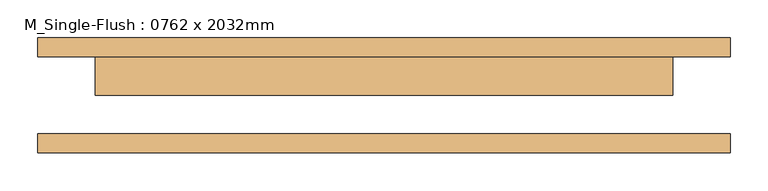
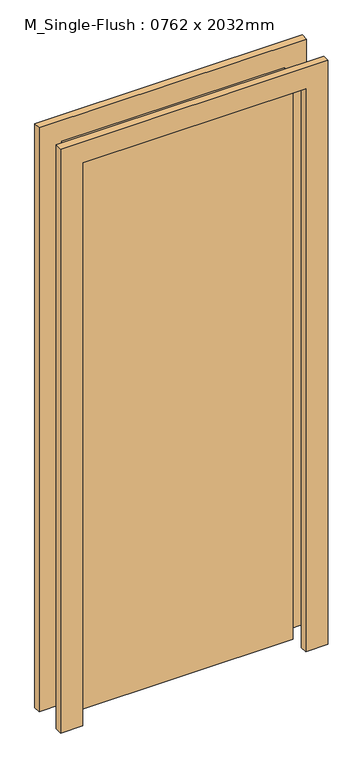
"""IFC4 building model written with IfcOpenShell, lengths in millimetres: door geometry, M_Single-Flush : 0762 x 2032mm."""

from ifc_helpers import new_model, si_unit, frame, origin, origin_with_axes, place, context, project, spatial, polyline, outline, extrude, source, transform, mapped, element, save


def m_single_flush_0762_x_2032mm_debabc81(model_context):
    return source(origin(), model_context, "Body", "SweptSolid", [
        extrude(outline(polyline([(2108.0, -457.0), (0.0, -457.0), (0.0, -381.0), (2032.0, -381.0), (2032.0, 381.0), (0.0, 381.0), (0.0, 457.0), (2108.0, 457.0), (2108.0, -457.0)])), frame((0.0, 50.8, 0.0), z_axis=(0.0, 1.0, 0.0), x_axis=(0.0, 0.0, 1.0)), (0.0, 0.0, 1.0), 25.0),
        extrude(outline(polyline([(2108.0, 457.0), (2108.0, -457.0), (0.0, -457.0), (0.0, -381.0), (2032.0, -381.0), (2032.0, 381.0), (0.0, 381.0), (0.0, 457.0), (2108.0, 457.0)])), frame((0.0, -75.8, 0.0), z_axis=(0.0, 1.0, 0.0), x_axis=(0.0, 0.0, 1.0)), (0.0, 0.0, 1.0), 25.0),
        extrude(outline(polyline([(381.0, -0.2), (-381.0, -0.2), (-381.0, 50.8), (381.0, 50.8), (381.0, -0.2)])), origin_with_axes(), (0.0, 0.0, 1.0), 2032.0),
    ])


if __name__ == "__main__":
    model = new_model("IFC4")
    model_context = context("Model", 3, world=origin())
    ifc_project = project(units=[si_unit("LENGTHUNIT", "METRE", prefix="MILLI")], contexts=[model_context])
    site = spatial("IfcSite", under=ifc_project)
    building = spatial("IfcBuilding", under=site)
    placement = place(None, origin())
    m_single_flush_0762_x_2032mm_shape = m_single_flush_0762_x_2032mm_debabc81(model_context)
    element("IfcDoor", 1, ObjectType="M_Single-Flush : 0762 x 2032mm", at=placement, inside=building, context=model_context, shape_type="MappedRepresentation", body=[
        mapped(m_single_flush_0762_x_2032mm_shape, transform((0.0, 0.0, 0.0), x_axis=(1.0, 0.0, 0.0), y_axis=(0.0, 1.0, 0.0), z_axis=(0.0, 0.0, 1.0))),
    ])
    save(model, "model.ifc")

# Revit data of these elements
# Type "M_Single-Flush : 0762 x 2032mm"
#   Type Mark = "28"
#   Construction Type Id = "MDOOR"
#   Analytic Construction = "Metal"
#   Thickness = 0.167323 ft
#   Thermal Resistance (R) = 0.270117 (m²·K)/W
#   Heat Transfer Coefficient (U) = 3.7021 W/(m²·K)
#   Height = 6.666667 ft
#   Trim Projection Ext = 0.082021 ft
#   Trim Projection Int = 0.082021 ft
#   Trim Width = 0.249344 ft
#   Width = 2.5 ft
#   Define Thermal Properties by = 1
#   Define Thermal Properties by = 1
#   Door Material = Door - Panel
#   Frame Material = Door - Frame
#   Visual Light Transmittance = 0
#   Solar Heat Gain Coefficient = 0
#   Function = (empty or 0)
#   Wall Closure = (empty or 0)
# Element 1 (IfcDoor, "M_Single-Flush : 0762 x 2032mm")
#   Materials on its faces: "Door - Frame", "Door - Panel"
# Materials
#   "Door - Panel": class "Wood", colour RGB 210 159 95, transparency 0, Cost = 0
#   "Door - Frame": colour RGB 118 70 51, transparency 0, Cost = 0
